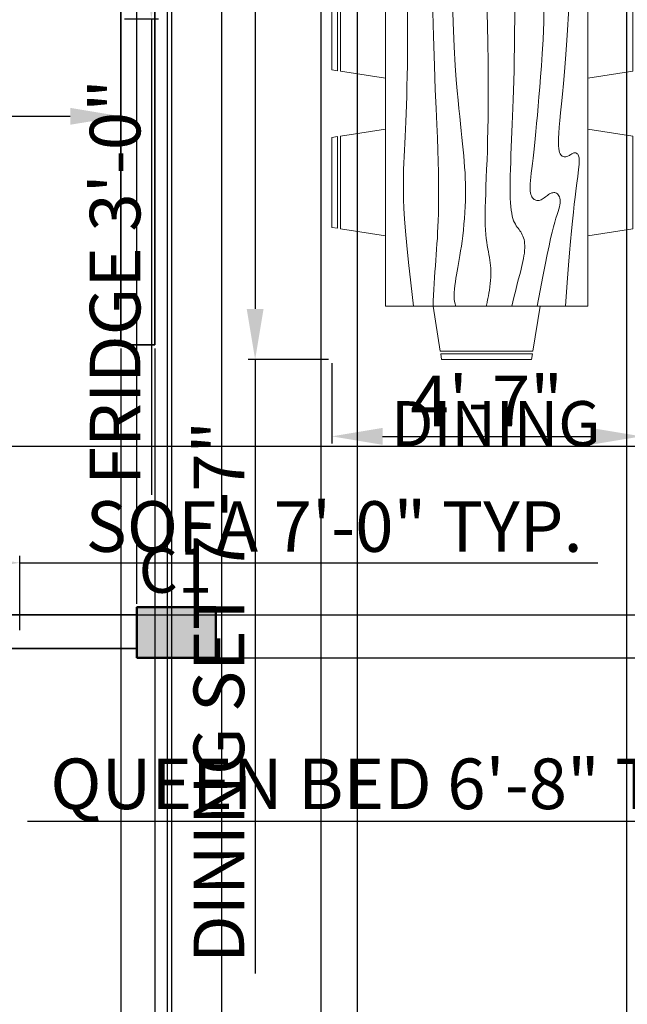
# Model space of a CAD drawing. Units: inches. Extents: x 2621 to 6190, y 513 to 1320.
# Tile 3 of 11: x 2889 to 2997, y 828 to 1003. Entities that reach past the tile are written whole.
import ezdxf

# ---------------------------------------------------------------- set-up
doc = ezdxf.new("R2010")
doc.units = ezdxf.units.IN
for name, color, linetype, lineweight in [('A-ANNO-DIMS', 5, 'Continuous', 18), ('A-AREA-IDEN', 7, 'Continuous', 25), ('A-WALL', 7, 'Continuous', 35), ('columns', 2, 'Continuous', 50), ('furniture', 30, 'Continuous', 18), ('S-COLS-IDEN', 2, 'Continuous', 25), ('S-COLS-PATT', 2, 'Continuous', 13)]:
    doc.layers.add(name, color=color, linetype=linetype, lineweight=lineweight)
doc.styles.get("Standard").update_dxf_attribs({"font": 'arial.ttf'})
doc.dimstyles.new('ISO-25', dxfattribs={"dimtxt": 9, "dimasz": 9, "dimexe": 1.25, "dimexo": 0.625, "dimtad": 1, "dimlunit": 3, "dimtxsty": 'Standard', "dimcen": 2.5, "dimadec": 0, "dimazin": 0, "dimtfac": 1, "dimtmove": 0, "dimatfit": 3, "dimfxl": 1, "dimarcsym": 0})

# ---------------------------------------------------------------- blocks, each defined once
blk = doc.blocks.new('Dining Set - 36 x 72 in.')
for p, q in [((-22, 27.5), (-22.1562, 26.50042)), ((-5.8416, 26.5), (-22.1534, 26.5)), ((-22, 27.5), (-6, 27.5)), ((-5.8437, 26.49966), (-6, 27.5)), ((6, 27.5), (5.8438, 26.50042)), ((22.1584, 26.5), (5.8466, 26.5)), ((6, 27.5), (22, 27.5)), ((22.1563, 26.49966), (22, 27.5)), ((-22.2343, 26.00059), (-23.4847, 17.99762)), ((-22.2304, 26), (-5.7608, 26)), ((-4.5152, 17.99762), (-5.7655, 25.99926)), ((5.7657, 26.00059), (4.5153, 17.99762)), ((5.7696, 26), (22.2392, 26)), ((23.4848, 17.99762), (22.2345, 25.99926)), ((36, 18), (-36, 18)), ((-36, 18), (-36, -18)), ((36, -18), (36, 18)), ((-44.0006, 8.23428), (-35.9976, 9.48474)), ((44.0006, 8.23428), (35.9976, 9.48474)), ((-45.5, 8), (-44.5004, 8.15617)), ((-45.5, 8), (-45.5, -8)), ((-44.5, -8.15843), (-44.5, 8.15338)), ((-44, 8.23041), (-44, -8.23915)), ((44, 8.23041), (44, -8.23915)), ((44.5, -8.15843), (44.5, 8.15338)), ((45.5, 8), (44.5005, 8.15617)), ((45.5, 8), (45.5, -8)), ((-44.4997, -8.15631), (-45.5, -8)), ((-35.9976, -9.48476), (-43.9993, -8.2345)), ((35.9976, -9.48476), (43.9993, -8.2345)), ((44.4997, -8.15631), (45.5, -8)), ((-36, -18), (36, -18)), ((-22.2343, -26.0006), (-23.4847, -17.99762)), ((-4.5152, -17.99762), (-5.7655, -25.99928)), ((5.7657, -26.0006), (4.5153, -17.99762)), ((23.4848, -17.99762), (22.2345, -25.99928)), ((-22.2304, -26), (-5.7608, -26)), ((5.7696, -26), (22.2392, -26)), ((-22, -27.5), (-22.1562, -26.50044)), ((-5.8416, -26.5), (-22.1534, -26.5)), ((-22, -27.5), (-6, -27.5)), ((-5.8437, -26.49967), (-6, -27.5)), ((6, -27.5), (5.8438, -26.50044)), ((22.1584, -26.5), (5.8466, -26.5)), ((6, -27.5), (22, -27.5)), ((22.1563, -26.49967), (22, -27.5))]:
    blk.add_line(p, q)
for points in [[(-36, 15), (-31.1772, 14.97754), (-26.8079, 14.91406), (-22.8538, 14.81543), (-19.276, 14.6875), (-16.0362, 14.53613), (-13.0957, 14.36718), (-10.4159, 14.18652), (-7.9583, 14), (-5.6904, 13.81315), (-3.6035, 13.63021), (-1.6954, 13.45508), (0.0365, 13.29166), (1.5945, 13.14388), (2.9811, 13.01562), (4.1988, 12.9108), (5.25, 12.83333), (6.1393, 12.78613), (6.8802, 12.76823), (7.4883, 12.77767), (7.9792, 12.8125), (8.3685, 12.87077), (8.6719, 12.95052), (8.9049, 13.0498), (9.0833, 13.16666), (9.2205, 13.29899), (9.3216, 13.44401), (9.3895, 13.59879), (9.4271, 13.76041), (9.4373, 13.92594), (9.4232, 14.09245), (9.3875, 14.257), (9.3333, 14.41666), (9.2638, 14.56917), (9.1836, 14.71484), (9.0975, 14.85465), (9.0104, 14.98958), (8.9272, 15.1206), (8.8529, 15.2487), (8.7922, 15.37483), (8.75, 15.5), (8.7305, 15.62467), (8.7344, 15.74739), (8.7617, 15.86621), (8.8125, 15.97916), (8.8867, 16.08431), (8.9844, 16.17968), (9.1055, 16.26334), (9.25, 16.33333), (9.4189, 16.38802), (9.6172, 16.42708), (9.8506, 16.45052), (10.125, 16.45833), (10.4463, 16.45052), (10.8203, 16.42708), (11.2529, 16.38802), (11.75, 16.33333), (12.3184, 16.26318), (12.9694, 16.17838), (13.7151, 16.07991), (14.5677, 15.96875), (15.5395, 15.84586), (16.6426, 15.71224), (17.8893, 15.56884), (19.2917, 15.41666), (20.859, 15.25667), (22.5879, 15.08984), (24.4721, 14.91715), (26.5052, 14.73958), (28.6809, 14.5581), (30.9929, 14.3737), (33.4347, 14.18733), (36, 14)], [(-36, 10), (-28.9766, 10.14274), (-23.1725, 10.20442), (-18.4241, 10.19775), (-14.5677, 10.13541), (-11.4399, 10.03011), (-8.877, 9.89453), (-6.7154, 9.74137), (-4.7917, 9.58333), (-2.9698, 9.43082), (-1.2246, 9.28515), (0.4415, 9.14534), (2.026, 9.01041), (3.5266, 8.87939), (4.9408, 8.7513), (6.266, 8.62516), (7.5, 8.5), (8.6411, 8.37549), (9.6914, 8.2539), (10.6538, 8.13818), (11.5312, 8.03125), (12.3267, 7.93603), (13.043, 7.85547), (13.6831, 7.79248), (14.25, 7.75), (14.7471, 7.7303), (15.1797, 7.73307), (15.5537, 7.75732), (15.875, 7.80208), (16.1494, 7.86637), (16.3828, 7.94922), (16.5811, 8.04964), (16.75, 8.16666), (16.8944, 8.29915), (17.0143, 8.44531), (17.1089, 8.60319), (17.1771, 8.77083), (17.218, 8.94629), (17.2305, 9.1276), (17.2137, 9.31282), (17.1667, 9.5), (17.0895, 9.6875), (16.987, 9.875), (16.8649, 10.0625), (16.7292, 10.25), (16.5856, 10.4375), (16.4401, 10.625), (16.2985, 10.8125), (16.1667, 11), (16.05, 11.18733), (15.9518, 11.3737), (15.8752, 11.5581), (15.8229, 11.73958), (15.798, 11.91715), (15.8034, 12.08984), (15.842, 12.25667), (15.9167, 12.41666), (16.0295, 12.56836), (16.1784, 12.70833), (16.3605, 12.83268), (16.5729, 12.9375), (16.8127, 13.01888), (17.0768, 13.07291), (17.3625, 13.0957), (17.6667, 13.08333), (17.9894, 13.03312), (18.3418, 12.94726), (18.7382, 12.82918), (19.1927, 12.68229), (19.7195, 12.51001), (20.3327, 12.31575), (21.0465, 12.10294), (21.875, 11.875), (22.8357, 11.63354), (23.959, 11.37304), (25.2786, 11.08618), (26.8282, 10.76562), (28.6414, 10.40405), (30.752, 9.99414), (33.1936, 9.52856), (36, 9)], [(-36, 5.5), (-30.7157, 5.3348), (-26.069, 5.20963), (-21.9946, 5.11767), (-18.4271, 5.05208), (-15.3009, 5.00602), (-12.5508, 4.97265), (-10.1112, 4.94515), (-7.9167, 4.91666), (-5.909, 4.88167), (-4.0586, 4.83984), (-2.3429, 4.79215), (-0.7396, 4.73958), (0.7739, 4.6831), (2.22, 4.6237), (3.6213, 4.56233), (5, 4.5), (6.373, 4.43782), (7.7344, 4.3776), (9.0723, 4.32129), (10.375, 4.27083), (11.6309, 4.22819), (12.8281, 4.19531), (13.9551, 4.17415), (15, 4.16666), (15.954, 4.17448), (16.819, 4.19791), (17.6001, 4.23698), (18.3021, 4.29166), (18.9299, 4.36198), (19.4883, 4.44791), (19.9823, 4.54948), (20.4167, 4.66666), (20.7969, 4.79899), (21.1302, 4.94401), (21.4245, 5.09879), (21.6875, 5.26041), (21.9271, 5.42594), (22.1511, 5.59245), (22.3672, 5.757), (22.5834, 5.91666), (22.8065, 6.06868), (23.0404, 6.21093), (23.2879, 6.34147), (23.5521, 6.45833), (23.8358, 6.55957), (24.142, 6.64323), (24.4735, 6.70735), (24.8334, 6.75), (25.2235, 6.76969), (25.642, 6.76692), (26.0858, 6.74267), (26.5521, 6.69791), (27.0379, 6.63362), (27.5404, 6.55078), (28.0565, 6.45036), (28.5834, 6.33333), (29.1242, 6.19987), (29.7071, 6.04687), (30.3661, 5.87044), (31.1354, 5.66666), (32.0493, 5.43164), (33.142, 5.16146), (34.4475, 4.85221), (36, 4.5)], [(-36, -1), (-30.7915, -0.6591), (-26.0195, -0.38216), (-21.6519, -0.16284), (-17.6563, 0.00521), (-14.0005, 0.12833), (-10.6523, 0.21289), (-7.5796, 0.26522), (-4.75, 0.29166), (-2.134, 0.29793), (0.2878, 0.28711), (2.5317, 0.26163), (4.6146, 0.22396), (6.5529, 0.17651), (8.3633, 0.12174), (10.0623, 0.06209), (11.6667, 0), (13.1899, -0.06201), (14.6341, -0.1211), (15.9982, -0.17432), (17.2813, -0.21875), (18.4823, -0.25147), (19.6003, -0.26953), (20.6343, -0.27002), (21.5834, -0.25), (22.4481, -0.20768), (23.2357, -0.14584), (23.9549, -0.06836), (24.6146, 0.02083), (25.2235, 0.11784), (25.7904, 0.21875), (26.3241, 0.31966), (26.8334, 0.41666), (27.3265, 0.50618), (27.8099, 0.58593), (28.2894, 0.65397), (28.7709, 0.70833), (29.2601, 0.74707), (29.763, 0.76823), (30.2855, 0.76985), (30.8334, 0.75), (31.4088, 0.70784), (31.9994, 0.64713), (32.589, 0.57275), (33.1615, 0.48958), (33.7008, 0.4025), (34.1908, 0.3164), (34.6153, 0.23616), (34.9584, 0.16666), (35.2099, 0.11165), (35.3848, 0.07031), (35.504, 0.04069), (35.5886, 0.02083), (35.6594, 0.00879), (35.7377, 0.0026), (35.8442, 0.00032), (36, 0)], [(-36, -6.5), (-27.1843, -6.31267), (-20.084, -6.1263), (-14.469, -5.9419), (-10.1094, -5.76042), (-6.7752, -5.58285), (-4.2363, -5.41016), (-2.2629, -5.24333), (-0.625, -5.08334), (0.8708, -4.93099), (2.2715, -4.78646), (3.5872, -4.64974), (4.8281, -4.52084), (6.0046, -4.39974), (7.127, -4.28646), (8.2053, -4.18099), (9.25, -4.08334), (10.2705, -3.99382), (11.2734, -3.91407), (12.2647, -3.84603), (13.25, -3.79167), (14.2354, -3.75293), (15.2266, -3.73177), (16.2295, -3.73015), (17.25, -3.75), (18.2912, -3.79248), (19.3451, -3.85547), (20.4009, -3.93604), (21.4479, -4.03125), (22.4754, -4.13819), (23.4727, -4.25391), (24.4289, -4.37549), (25.3334, -4.5), (26.1785, -4.62492), (26.9694, -4.74935), (27.7145, -4.87281), (28.4219, -4.99479), (29.1, -5.11483), (29.7572, -5.23242), (30.4016, -5.34709), (31.0417, -5.45834), (31.6837, -5.56437), (32.3262, -5.65821), (32.9658, -5.73153), (33.599, -5.77604), (34.2224, -5.78345), (34.8327, -5.74545), (35.4264, -5.65373), (36, -5.5)], [(-36, -10), (-26.4022, -9.81299), (-18.4675, -9.62891), (-11.9839, -9.45069), (-6.7396, -9.28125), (-2.5226, -9.12354), (0.8789, -8.98047), (3.6769, -8.85498), (6.0833, -8.75), (8.2767, -8.66765), (10.3021, -8.60677), (12.1712, -8.56543), (13.8958, -8.54167), (15.4876, -8.53353), (16.9583, -8.53907), (18.3197, -8.55632), (19.5834, -8.58334), (20.7616, -8.61841), (21.8685, -8.66081), (22.9188, -8.71004), (23.9271, -8.76563), (24.9081, -8.82707), (25.8763, -8.89388), (26.8465, -8.96558), (27.8334, -9.04167), (28.8474, -9.12118), (29.8828, -9.20117), (30.93, -9.27824), (31.9792, -9.34896), (33.0205, -9.40991), (34.0443, -9.45768), (35.0407, -9.48885), (36, -9.5)], [(-36, -14.5), (-30.0881, -14.33513), (-25.0332, -14.21224), (-20.7312, -14.12647), (-17.0781, -14.07292), (-13.97, -14.04671), (-11.3027, -14.04297), (-8.9724, -14.05681), (-6.875, -14.08334), (-4.9224, -14.11833), (-3.0905, -14.16016), (-1.3709, -14.20785), (0.2448, -14.26042), (1.7647, -14.3169), (3.1973, -14.3763), (4.5507, -14.43767), (5.8333, -14.5), (7.0554, -14.5621), (8.235, -14.62175), (9.3922, -14.67652), (10.5469, -14.72396), (11.7192, -14.76164), (12.929, -14.78711), (14.1965, -14.79794), (15.5417, -14.79167), (16.9933, -14.76424), (18.6152, -14.70508), (20.4804, -14.60197), (22.6615, -14.44271), (25.2312, -14.21509), (28.2624, -13.9069), (31.8277, -13.50594), (36, -13)]]:
    blk.add_lwpolyline(points)
blk = doc.blocks.new('*D19')
at = {"layer": 'A-ANNO-DIMS', "color": 0, "lineweight": -2, "transparency": 16777216}
for p, q in [((2787.38, 984.93), (2787.38, 984.3)), ((2796.38, 985.55), (2898.38, 985.55)), ((2907.38, 984.93), (2907.38, 984.3))]:
    blk.add_line(p, q, dxfattribs=at)
at = {"layer": 'A-ANNO-DIMS', "color": 0, "transparency": 16777216}
for points in [[(2796.38, 987.05), (2796.38, 984.05), (2787.38, 985.55)], [(2898.38, 987.05), (2898.38, 984.05), (2907.38, 985.55)]]:
    blk.add_solid(points, dxfattribs=at)
at = {"layer": 'Defpoints', "color": 0, "transparency": 16777216}
for p in [(2787.38, 985.55), (2907.38, 985.55), (2907.38, 985.55)]:
    blk.add_point(p, dxfattribs=at)
at = {"layer": 'A-ANNO-DIMS', "color": 0, "transparency": 16777216, "insert": (2847.38, 990.77), "char_height": 9, "attachment_point": 5}
blk.add_mtext("10'", dxfattribs=at)
blk = doc.blocks.new('COL-C1-9X14')
blk.add_lwpolyline([(0, 0), (0, 9), (14, 9), (14, 0)], close=True)
blk = doc.blocks.new('*D63')
at = {"layer": 'A-ANNO-DIMS', "color": 0, "lineweight": -2, "transparency": 16777216}
for p, q in [((3033.38, 860.14), (2890.74, 860.14)), ((3033.38, 848.76), (3033.38, 861.39)), ((3104.38, 860.14), (3042.38, 860.14)), ((3113.38, 848.76), (3113.38, 861.39))]:
    blk.add_line(p, q, dxfattribs=at)
at = {"layer": 'A-ANNO-DIMS', "color": 0, "transparency": 16777216}
for points in [[(3042.38, 861.64), (3042.38, 858.64), (3033.38, 860.14)], [(3104.38, 861.64), (3104.38, 858.64), (3113.38, 860.14)]]:
    blk.add_solid(points, dxfattribs=at)
at = {"layer": 'Defpoints', "color": 0, "transparency": 16777216}
for p in [(3033.38, 860.14), (3033.38, 848.14), (3113.38, 848.14)]:
    blk.add_point(p, dxfattribs=at)
at = {"layer": 'A-ANNO-DIMS', "color": 0, "transparency": 16777216, "insert": (2957.56, 865.69), "char_height": 9, "attachment_point": 5}
blk.add_mtext('QUEEN BED 6\'-8" TYP.', dxfattribs=at)
blk = doc.blocks.new('*D65')
at = {"layer": 'A-ANNO-DIMS', "color": 0, "lineweight": -2, "transparency": 16777216}
for p, q in [((2805.38, 894.18), (2805.38, 907.41)), ((2889.38, 894.18), (2889.38, 907.41)), ((2814.38, 906.16), (2880.38, 906.16)), ((2889.38, 906.16), (2992.17, 906.16))]:
    blk.add_line(p, q, dxfattribs=at)
at = {"layer": 'A-ANNO-DIMS', "color": 0, "transparency": 16777216}
for points in [[(2814.38, 907.66), (2814.38, 904.66), (2805.38, 906.16)], [(2880.38, 907.66), (2880.38, 904.66), (2889.38, 906.16)]]:
    blk.add_solid(points, dxfattribs=at)
at = {"layer": 'Defpoints', "color": 0, "transparency": 16777216}
for p in [(2889.38, 906.16), (2805.38, 893.56), (2889.38, 893.56)]:
    blk.add_point(p, dxfattribs=at)
at = {"layer": 'A-ANNO-DIMS', "color": 0, "transparency": 16777216, "insert": (2945.28, 911.44), "char_height": 9, "attachment_point": 5}
blk.add_mtext('SOFA 7\'-0" TYP.', dxfattribs=at)
blk = doc.blocks.new('*D73')
at = {"layer": 'A-ANNO-DIMS', "color": 0, "lineweight": -2, "transparency": 16777216}
for p, q in [((2944.26, 1033.29), (2929.98, 1033.29)), ((2931.23, 1024.29), (2931.23, 951.29)), ((2944.26, 942.29), (2929.98, 942.29)), ((2931.23, 942.29), (2931.23, 833.12))]:
    blk.add_line(p, q, dxfattribs=at)
at = {"layer": 'A-ANNO-DIMS', "color": 0, "transparency": 16777216}
for points in [[(2929.73, 1024.29), (2932.73, 1024.29), (2931.23, 1033.29)], [(2929.73, 951.29), (2932.73, 951.29), (2931.23, 942.29)]]:
    blk.add_solid(points, dxfattribs=at)
at = {"layer": 'Defpoints', "color": 0, "transparency": 16777216}
for p in [(2944.88, 1033.29), (2931.23, 942.29), (2944.88, 942.29)]:
    blk.add_point(p, dxfattribs=at)
at = {"layer": 'A-ANNO-DIMS', "color": 0, "transparency": 16777216, "insert": (2925.95, 883.21), "char_height": 9, "attachment_point": 5, "rotation": 90}
blk.add_mtext('DINING SET 7\'-7"', dxfattribs=at)
blk = doc.blocks.new('*D74')
at = {"layer": 'A-ANNO-DIMS', "color": 0, "lineweight": -2, "transparency": 16777216}
for p, q in [((2944.88, 941.67), (2944.88, 927.39)), ((2999.88, 941.67), (2999.88, 927.39)), ((2953.88, 928.64), (2990.88, 928.64))]:
    blk.add_line(p, q, dxfattribs=at)
at = {"layer": 'A-ANNO-DIMS', "color": 0, "transparency": 16777216}
for points in [[(2953.88, 930.14), (2953.88, 927.14), (2944.88, 928.64)], [(2990.88, 930.14), (2990.88, 927.14), (2999.88, 928.64)]]:
    blk.add_solid(points, dxfattribs=at)
at = {"layer": 'Defpoints', "color": 0, "transparency": 16777216}
for p in [(2944.88, 942.29), (2999.88, 942.29), (2999.88, 928.64)]:
    blk.add_point(p, dxfattribs=at)
at = {"layer": 'A-ANNO-DIMS', "color": 0, "transparency": 16777216, "insert": (2972.38, 933.77), "char_height": 9, "attachment_point": 5}
blk.add_mtext('4\'-7"', dxfattribs=at)
blk = doc.blocks.new('*D75')
at = {"layer": 'A-ANNO-DIMS', "color": 0, "lineweight": -2, "transparency": 16777216}
for p, q in [((2908.01, 1038.89), (2914.03, 1038.89)), ((2912.78, 1029.89), (2912.78, 1011.89)), ((2908.01, 1002.89), (2914.03, 1002.89)), ((2912.78, 1002.89), (2912.78, 918.24))]:
    blk.add_line(p, q, dxfattribs=at)
at = {"layer": 'A-ANNO-DIMS', "color": 0, "transparency": 16777216}
for points in [[(2911.28, 1029.89), (2914.28, 1029.89), (2912.78, 1038.89)], [(2911.28, 1011.89), (2914.28, 1011.89), (2912.78, 1002.89)]]:
    blk.add_solid(points, dxfattribs=at)
at = {"layer": 'Defpoints', "color": 0, "transparency": 16777216}
for p in [(2907.38, 1038.89), (2907.38, 1002.89), (2912.78, 1002.89)]:
    blk.add_point(p, dxfattribs=at)
at = {"layer": 'A-ANNO-DIMS', "color": 0, "transparency": 16777216, "insert": (2907.5, 956.07), "char_height": 9, "attachment_point": 5, "rotation": 90}
blk.add_mtext('FRIDGE 3\'-0"', dxfattribs=at)
blk = doc.blocks.new('*D82')
at = {"layer": 'A-ANNO-DIMS', "color": 0, "lineweight": -2, "transparency": 16777216}
for p, q in [((2924.85, 889.24), (3291.63, 889.24)), ((3290.38, 719.89), (3290.38, 880.24)), ((2917.49, 710.89), (3291.63, 710.89))]:
    blk.add_line(p, q, dxfattribs=at)
at = {"layer": 'A-ANNO-DIMS', "color": 0, "transparency": 16777216}
for points in [[(3288.88, 880.24), (3291.88, 880.24), (3290.38, 889.24)], [(3288.88, 719.89), (3291.88, 719.89), (3290.38, 710.89)]]:
    blk.add_solid(points, dxfattribs=at)
at = {"layer": 'Defpoints', "color": 0, "transparency": 16777216}
for p in [(2924.22, 889.24), (3290.38, 889.24), (2916.87, 710.89)]:
    blk.add_point(p, dxfattribs=at)
at = {"layer": 'A-ANNO-DIMS', "color": 0, "transparency": 16777216, "insert": (3285.1, 800.07), "char_height": 9, "attachment_point": 5, "rotation": 90}
blk.add_mtext('14\'-10 1/2"', dxfattribs=at)
blk = doc.blocks.new('*D87')
at = {"layer": 'A-ANNO-DIMS', "color": 0, "lineweight": -2, "transparency": 16777216}
for p, q in [((2778.38, 897.51), (2778.38, 1155.14)), ((2787.38, 1153.89), (2901.22, 1153.89)), ((2910.22, 898.87), (2910.22, 1155.14))]:
    blk.add_line(p, q, dxfattribs=at)
at = {"layer": 'A-ANNO-DIMS', "color": 0, "transparency": 16777216}
for points in [[(2787.38, 1155.39), (2787.38, 1152.39), (2778.38, 1153.89)], [(2901.22, 1155.39), (2901.22, 1152.39), (2910.22, 1153.89)]]:
    blk.add_solid(points, dxfattribs=at)
at = {"layer": 'Defpoints', "color": 0, "transparency": 16777216}
for p in [(2910.22, 1153.89), (2910.22, 898.24), (2778.38, 896.89)]:
    blk.add_point(p, dxfattribs=at)
at = {"layer": 'A-ANNO-DIMS', "color": 0, "transparency": 16777216, "insert": (2844.3, 1159.11), "char_height": 9, "attachment_point": 5}
blk.add_mtext('11\'-0"', dxfattribs=at)
blk = doc.blocks.new('*D88')
at = {"layer": 'A-ANNO-DIMS', "color": 0, "lineweight": -2, "transparency": 16777216}
for p, q in [((2910.22, 898.87), (2910.22, 1155.14)), ((2919.22, 1153.89), (3018.38, 1153.89)), ((3027.38, 898.01), (3027.38, 1155.14))]:
    blk.add_line(p, q, dxfattribs=at)
at = {"layer": 'A-ANNO-DIMS', "color": 0, "transparency": 16777216}
for points in [[(2919.22, 1155.39), (2919.22, 1152.39), (2910.22, 1153.89)], [(3018.38, 1155.39), (3018.38, 1152.39), (3027.38, 1153.89)]]:
    blk.add_solid(points, dxfattribs=at)
at = {"layer": 'Defpoints', "color": 0, "transparency": 16777216}
for p in [(3027.38, 1153.89), (2910.22, 898.24), (3027.38, 897.39)]:
    blk.add_point(p, dxfattribs=at)
at = {"layer": 'A-ANNO-DIMS', "color": 0, "transparency": 16777216, "insert": (2968.8, 1159.11), "char_height": 9, "attachment_point": 5}
blk.add_mtext('9\'-9"', dxfattribs=at)
blk = doc.blocks.new('*D94')
at = {"layer": 'A-ANNO-DIMS', "color": 0, "lineweight": -2, "transparency": 16777216}
for p, q in [((2925.32, 711.51), (2925.32, 1155.14)), ((2934.32, 1153.89), (2988.32, 1153.89)), ((2997.32, 711.51), (2997.32, 1155.14))]:
    blk.add_line(p, q, dxfattribs=at)
at = {"layer": 'A-ANNO-DIMS', "color": 0, "transparency": 16777216}
for points in [[(2934.32, 1155.39), (2934.32, 1152.39), (2925.32, 1153.89)], [(2988.32, 1155.39), (2988.32, 1152.39), (2997.32, 1153.89)]]:
    blk.add_solid(points, dxfattribs=at)
at = {"layer": 'Defpoints', "color": 0, "transparency": 16777216}
for p in [(2997.32, 1153.89), (2925.32, 710.89), (2997.32, 710.89)]:
    blk.add_point(p, dxfattribs=at)
at = {"layer": 'A-ANNO-DIMS', "color": 0, "transparency": 16777216, "insert": (2961.32, 1159.11), "char_height": 9, "attachment_point": 5}
blk.add_mtext('6\'-0"', dxfattribs=at)
blk = doc.blocks.new('*D100')
at = {"layer": 'A-ANNO-DIMS', "color": 0, "lineweight": -2, "transparency": 16777216}
for p, q in [((2854.01, 926.89), (3291.63, 926.89)), ((3290.38, 905.89), (3290.38, 917.89)), ((2854.01, 896.89), (3291.63, 896.89))]:
    blk.add_line(p, q, dxfattribs=at)
at = {"layer": 'A-ANNO-DIMS', "color": 0, "transparency": 16777216}
for points in [[(3288.88, 917.89), (3291.88, 917.89), (3290.38, 926.89)], [(3288.88, 905.89), (3291.88, 905.89), (3290.38, 896.89)]]:
    blk.add_solid(points, dxfattribs=at)
at = {"layer": 'Defpoints', "color": 0, "transparency": 16777216}
for p in [(2853.38, 926.89), (3290.38, 926.89), (2853.38, 896.89)]:
    blk.add_point(p, dxfattribs=at)
at = {"layer": 'A-ANNO-DIMS', "color": 0, "transparency": 16777216, "insert": (3285.16, 911.89), "char_height": 9, "attachment_point": 5, "rotation": 90}
blk.add_mtext('2\'-6"', dxfattribs=at)
blk = doc.blocks.new('*D101')
at = {"layer": 'A-ANNO-DIMS', "color": 0, "lineweight": -2, "transparency": 16777216}
for p, q in [((2907.38, 944.26), (2907.38, 519.64)), ((2913.38, 944.26), (2913.38, 519.64)), ((2898.38, 520.89), (2889.38, 520.89)), ((2907.38, 520.89), (2913.38, 520.89)), ((2922.38, 520.89), (2956.56, 520.89))]:
    blk.add_line(p, q, dxfattribs=at)
at = {"layer": 'A-ANNO-DIMS', "color": 0, "transparency": 16777216}
for points in [[(2898.38, 522.39), (2898.38, 519.39), (2907.38, 520.89)], [(2922.38, 522.39), (2922.38, 519.39), (2913.38, 520.89)]]:
    blk.add_solid(points, dxfattribs=at)
at = {"layer": 'Defpoints', "color": 0, "transparency": 16777216}
for p in [(2907.38, 944.89), (2913.38, 944.89), (2913.38, 520.89)]:
    blk.add_point(p, dxfattribs=at)
at = {"layer": 'A-ANNO-DIMS', "color": 0, "transparency": 16777216, "insert": (2943.97, 526.11), "char_height": 9, "attachment_point": 5}
blk.add_mtext('0\'-6"', dxfattribs=at)
blk = doc.blocks.new('*D102')
at = {"layer": 'A-ANNO-DIMS', "color": 0, "lineweight": -2, "transparency": 16777216}
for p, q in [((2915.57, 1054.4), (2915.57, 519.64)), ((2942.88, 1054.4), (2942.88, 519.64)), ((2924.57, 520.89), (2933.88, 520.89)), ((2942.88, 520.89), (2998.18, 520.89))]:
    blk.add_line(p, q, dxfattribs=at)
at = {"layer": 'A-ANNO-DIMS', "color": 0, "transparency": 16777216}
for points in [[(2924.57, 522.39), (2924.57, 519.39), (2915.57, 520.89)], [(2933.88, 522.39), (2933.88, 519.39), (2942.88, 520.89)]]:
    blk.add_solid(points, dxfattribs=at)
at = {"layer": 'Defpoints', "color": 0, "transparency": 16777216}
for p in [(2915.57, 1055.03), (2942.88, 1055.03), (2942.88, 520.89)]:
    blk.add_point(p, dxfattribs=at)
at = {"layer": 'A-ANNO-DIMS', "color": 0, "transparency": 16777216, "insert": (2975.03, 526.17), "char_height": 9, "attachment_point": 5}
blk.add_mtext('2\'-3 1/2"', dxfattribs=at)
blk = doc.blocks.new('*D106')
at = {"layer": 'A-ANNO-DIMS', "color": 0, "lineweight": -2, "transparency": 16777216}
for p, q in [((2949.38, 1076.26), (2949.38, 519.64)), ((2916.38, 1071.26), (2916.38, 519.64)), ((2925.38, 520.89), (2940.38, 520.89))]:
    blk.add_line(p, q, dxfattribs=at)
at = {"layer": 'A-ANNO-DIMS', "color": 0, "transparency": 16777216}
for points in [[(2925.38, 522.39), (2925.38, 519.39), (2916.38, 520.89)], [(2940.38, 522.39), (2940.38, 519.39), (2949.38, 520.89)]]:
    blk.add_solid(points, dxfattribs=at)
at = {"layer": 'Defpoints', "color": 0, "transparency": 16777216}
for p in [(2949.38, 1076.89), (2916.38, 1071.89), (2949.38, 520.89)]:
    blk.add_point(p, dxfattribs=at)
at = {"layer": 'A-ANNO-DIMS', "color": 0, "transparency": 16777216, "insert": (2932.88, 526.11), "char_height": 9, "attachment_point": 5}
blk.add_mtext('2\'-9"', dxfattribs=at)

msp = doc.modelspace()

# ---------------------------------------------------------------- hatches: boundary and pattern name
at = {"layer": 'S-COLS-PATT'}
h = msp.add_hatch(color=256, dxfattribs=at)
h.dxf.hatch_style = 1
h.paths.add_polyline_path([(2787.381, 1085.89), (2778.381, 1085.89), (2778.381, 1071.89), (2787.381, 1071.89)])
h.paths.add_polyline_path([(3222.381, 1085.89), (3208.381, 1085.89), (3208.381, 1076.89), (3222.381, 1076.89)])
h.paths.add_polyline_path([(3041.381, 1085.89), (3027.381, 1085.89), (3027.381, 1076.89), (3041.381, 1076.89)])
h.paths.add_polyline_path([(2916.381, 1085.89), (2907.381, 1085.89), (2907.381, 1076.89), (2916.381, 1076.89)])
h.paths.add_polyline_path([(2916.381, 1076.89), (2913.381, 1076.89), (2913.381, 1071.89), (2916.381, 1071.89)])
h.paths.add_polyline_path([(2913.381, 1076.89), (2907.381, 1076.89), (2907.381, 1071.89), (2913.381, 1071.89)])
h.paths.add_polyline_path([(2787.381, 896.89), (2778.381, 896.89), (2778.381, 882.89), (2787.381, 882.89)])
h.paths.add_polyline_path([(2924.221, 898.241), (2910.221, 898.241), (2910.221, 889.241), (2924.221, 889.241)])
h.paths.add_polyline_path([(3036.381, 896.89), (3033.381, 896.89), (3027.381, 897.385), (3027.381, 883.385), (3033.381, 883.385), (3033.381, 890.89), (3036.381, 890.89)])
h.paths.add_polyline_path([(3036.381, 890.89), (3033.381, 890.89), (3033.381, 883.385), (3036.381, 883.385)], flags=17)
h.paths.add_polyline_path([(3222.381, 897.745), (3213.381, 897.745), (3213.381, 883.745), (3222.381, 883.745)])
h.paths.add_polyline_path([(3222.381, 710.89), (3208.381, 710.89), (3208.381, 701.89), (3222.381, 701.89)])
h.paths.add_polyline_path([(3039.318, 710.89), (3021.318, 710.89), (3021.318, 701.89), (3039.318, 701.89)])
h.paths.add_polyline_path([(2796.381, 710.89), (2778.381, 710.89), (2778.381, 701.89), (2796.381, 701.89)])

# ---------------------------------------------------------------- linework, layer by layer
at = {"layer": 'A-WALL'}
for p, q in [((2907.381, 1076.89), (2907.381, 944.89)), ((2913.381, 1071.89), (2913.381, 944.89)), ((2913.381, 944.89), (2907.381, 944.89)), ((2907.381, 896.89), (2787.381, 896.89)), ((2910.221, 896.89), (2907.381, 896.89)), ((2907.381, 890.89), (2787.381, 890.89)), ((2910.221, 890.89), (2907.381, 890.89))]:
    msp.add_line(p, q, dxfattribs=at)

# ---------------------------------------------------------------- block references
at = {"layer": 'columns'}
msp.add_blockref('COL-C1-9X14', (2910.221, 889.241), dxfattribs=at)
at = {"layer": 'furniture', "rotation": 270}
msp.add_blockref('Dining Set - 36 x 72 in.', (2972.381, 987.791), dxfattribs=at)

# ---------------------------------------------------------------- texts
at = {"layer": 'A-AREA-IDEN', "insert": (2955.418, 934.907), "char_height": 8, "attachment_point": 1}
msp.add_mtext_dynamic_manual_height_columns('DINING ', width=40.12902, gutter_width=12.5, heights=[0], dxfattribs=at)
at = {"layer": 'S-COLS-IDEN', "insert": (2910.532, 908.828), "char_height": 8, "attachment_point": 1}
msp.add_mtext_dynamic_manual_height_columns('C1', width=53.01391, gutter_width=12.5, heights=[0], dxfattribs=at)

# ---------------------------------------------------------------- dimensions: what is measured, and where the dimension line sits
at = {"layer": 'A-ANNO-DIMS'}
for base, p1, p2, override, picture, middle in [((2910.221, 1153.89), (2778.381, 896.89), (2910.221, 898.241), {"dimdec": 1, "dimlfac": 1, "dimrnd": 0, "dimzin": 1, "dimdsep": 46, "dimlunit": 4, "dimfrac": 2}, '*D87', (2844.301, 1159.11)), ((3027.381, 1153.89), (2910.221, 898.241), (3027.381, 897.385), {"dimdec": 1, "dimlfac": 1, "dimrnd": 0, "dimzin": 1, "dimdsep": 46, "dimlunit": 4, "dimfrac": 2}, '*D88', (2968.801, 1159.11)), ((2997.318, 1153.89), (2925.318, 710.89), (2997.318, 710.89), {"dimdec": 1, "dimlfac": 1, "dimrnd": 0, "dimzin": 1, "dimdsep": 46, "dimlunit": 4, "dimfrac": 2}, '*D94', (2961.318, 1159.11)), ((2949.381, 520.89), (2916.381, 1071.89), (2949.381, 1076.89), {"dimdec": 1, "dimlfac": 1, "dimrnd": 0, "dimzin": 1, "dimdsep": 46, "dimlunit": 4, "dimfrac": 2}, '*D106', (2932.881, 526.11)), ((2942.877, 520.89), (2915.573, 1055.025), (2942.877, 1055.025), {"dimdec": 1, "dimlfac": 1, "dimrnd": 0, "dimzin": 1, "dimdsep": 46, "dimlunit": 4, "dimfrac": 2}, '*D102', (2975.027, 526.171)), ((2907.381, 985.551), (2787.381, 985.551), (2907.381, 985.551), {"dimclrd": 0, "dimclre": 0, "dimclrt": 0}, '*D19', (2847.381, 990.771)), ((2913.381, 520.89), (2907.381, 944.89), (2913.381, 944.89), {"dimdec": 1, "dimlfac": 1, "dimrnd": 0, "dimzin": 1, "dimdsep": 46, "dimlunit": 4, "dimfrac": 2}, '*D101', (2943.968, 526.11)), ((2999.881, 928.641), (2944.881, 942.291), (2999.881, 942.291), {"dimdec": 1, "dimlfac": 1, "dimrnd": 0, "dimzin": 1, "dimdsep": 46, "dimlunit": 4, "dimfrac": 2}, '*D74', (2972.381, 933.766))]:
    dim = msp.add_linear_dim(base=base, p1=p1, p2=p2, dimstyle='ISO-25', override=override, dxfattribs=at)
    dim.commit()
    dim.dimension.update_dxf_attribs({"geometry": picture, "text_midpoint": middle})
for base, p1, p2, angle, text, picture, middle in [((2912.781, 1002.894), (2907.381, 1038.894), (2907.381, 1002.894), 270, 'FRIDGE <>', '*D75', (2907.499, 956.066)), ((2931.231, 942.291), (2944.881, 1033.291), (2944.881, 942.291), 270, 'DINING SET <>', '*D73', (2925.952, 883.206)), ((3033.381, 860.137), (3113.381, 848.137), (3033.381, 848.137), 180, 'QUEEN BED <> TYP.', '*D63', (2957.561, 865.692))]:
    dim = msp.add_linear_dim(base=base, p1=p1, p2=p2, angle=angle, text=text, dimstyle='ISO-25', override={"dimdec": 1, "dimlfac": 1, "dimrnd": 0, "dimzin": 1, "dimdsep": 46, "dimlunit": 4, "dimfrac": 2}, dxfattribs=at)
    dim.commit()
    dim.dimension.update_dxf_attribs({"geometry": picture, "text_midpoint": middle})
dim = msp.add_linear_dim(base=(2889.381, 906.156), p1=(2805.381, 893.556), p2=(2889.381, 893.556), text='SOFA <> TYP.', dimstyle='ISO-25', override={"dimdec": 1, "dimlfac": 1, "dimrnd": 0, "dimzin": 1, "dimdsep": 46, "dimlunit": 4, "dimfrac": 2}, dxfattribs=at)
dim.commit()
dim.dimension.update_dxf_attribs({"geometry": '*D65', "text_midpoint": (2945.277, 911.438)})
for base, p1, p2, picture, middle in [((3290.381, 926.89), (2853.381, 896.89), (2853.381, 926.89), '*D100', (3285.161, 911.89)), ((3290.381, 889.241), (2916.869, 710.89), (2924.221, 889.241), '*D82', (3285.103, 800.065))]:
    dim = msp.add_linear_dim(base=base, p1=p1, p2=p2, angle=90, dimstyle='ISO-25', override={"dimdec": 1, "dimlfac": 1, "dimrnd": 0, "dimzin": 1, "dimdsep": 46, "dimlunit": 4, "dimfrac": 2}, dxfattribs=at)
    dim.commit()
    dim.dimension.update_dxf_attribs({"geometry": picture, "text_midpoint": middle})

doc.saveas('drawing.dxf')
